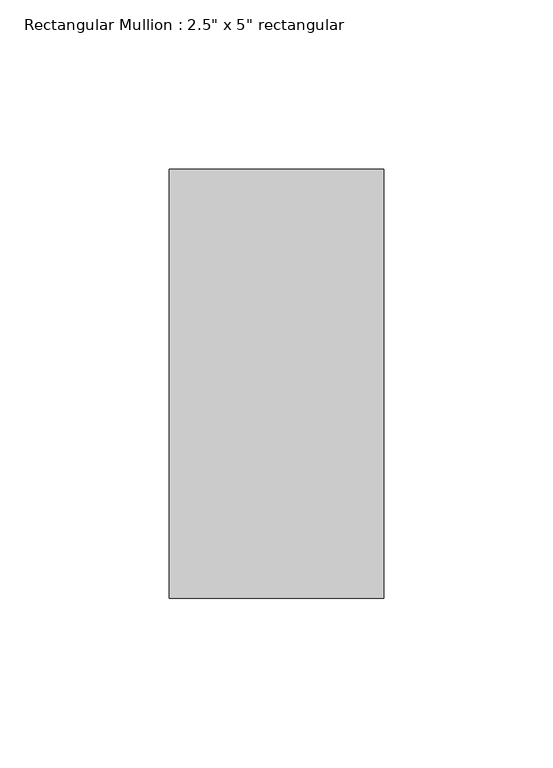
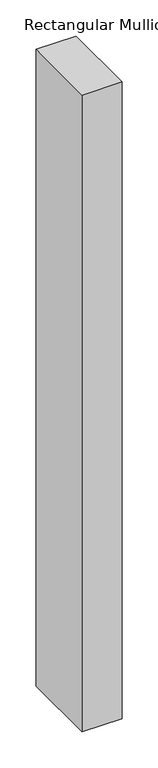
"""IFC4 building model written with IfcOpenShell, lengths in millimetres: member geometry."""

from ifc_helpers import new_model, si_unit, frame, origin, place, context, project, spatial, polyline, outline, extrude, source, transform, mapped, element, save


def member_4d6ef9b1(model_context):
    return source(origin(), model_context, "Body", "SweptSolid", [
        extrude(outline(polyline([(0.0, 63.5), (0.0, -63.5), (-63.5, -63.5), (-63.5, 63.5), (0.0, 63.5)])), frame((0.0, 0.0, -1073.15), z_axis=(0.0, 0.0, 1.0), x_axis=(1.0, 0.0, 0.0)), (0.0, 0.0, 1.0), 1073.15),
    ])


if __name__ == "__main__":
    model = new_model("IFC4")
    model_context = context("Model", 3, world=origin())
    ifc_project = project(units=[si_unit("LENGTHUNIT", "METRE", prefix="MILLI")], contexts=[model_context])
    site = spatial("IfcSite", under=ifc_project)
    building = spatial("IfcBuilding", under=site)
    placement = place(None, origin())
    member_shape = member_4d6ef9b1(model_context)
    element("IfcMember", 1, ObjectType="Rectangular Mullion : 2.5\" x 5\" rectangular", at=placement, inside=building, context=model_context, shape_type="MappedRepresentation", body=[
        mapped(member_shape, transform((0.0, 0.0, 0.0), x_axis=(1.0, 0.0, 0.0), y_axis=(0.0, 1.0, 0.0), z_axis=(0.0, 0.0, 1.0))),
    ])
    save(model, "model.ifc")

# Revit data of these elements
# Type "Rectangular Mullion : 2.5\" x 5\" rectangular"
#   built-in parameter 1007304 = 0.416667 (stored number, unit not read)
#   built-in parameter 1007301 = 0.104167 (stored number, unit not read)
#   built-in parameter 1007300 = 0.104167 (stored number, unit not read)
# Element 1 (IfcMember, "Rectangular Mullion : 2.5\" x 5\" rectangular")
#   Materials on its faces: "Iron, Ductile"
# Materials
#   "Iron, Ductile": class "Metal", colour RGB 0 0 0, transparency 0, Description = "Ductile cast iron", Cost = 0
